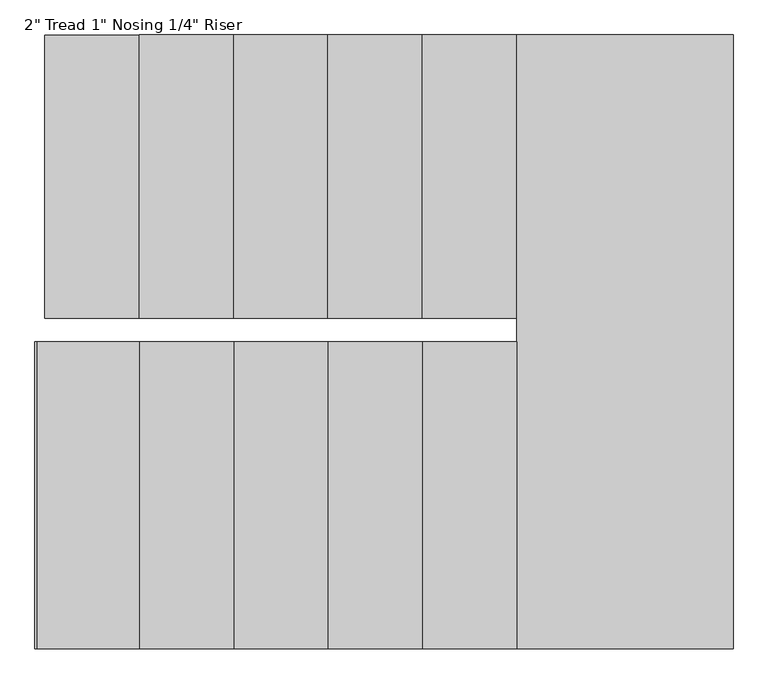
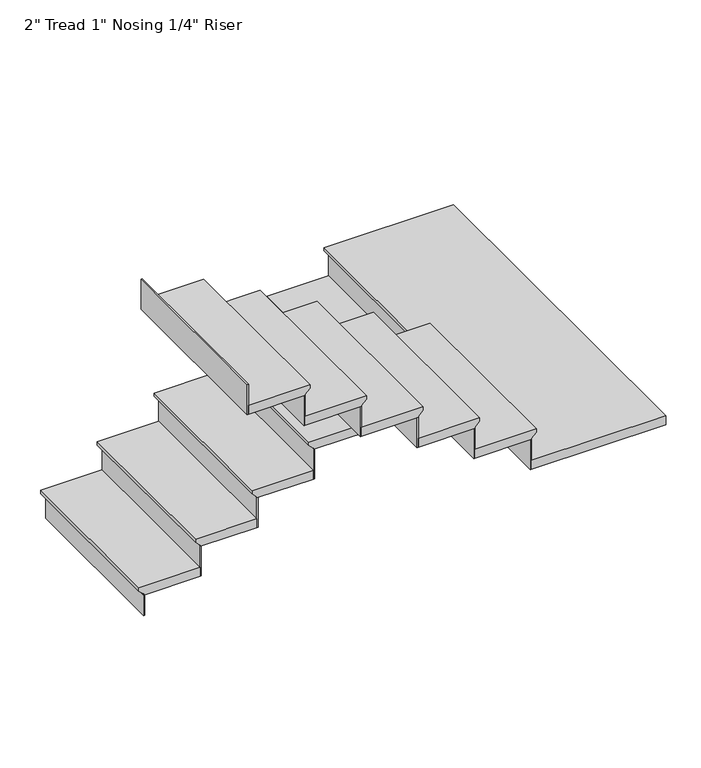
"""IFC4 building model written with IfcOpenShell, lengths in millimetres: stair flight geometry."""

from ifc_helpers import new_model, si_unit, origin, place, context, project, spatial, faceted_brep, source, transform, mapped, element, save


def stair_flight_f370bc99(model_context):
    return source(origin(), model_context, "Body", "Brep", [
        faceted_brep([(-1179.0415084, -2827.3064015, 6551.0833333), (-1179.0415084, -2827.3064015, 6570.1333333), (-1179.0415084, -1912.9064015, 6570.1333333), (-1179.0415084, -1912.9064015, 6551.0833333), (-1153.6415084, -2827.3064015, 6525.6833333), (-1153.6415084, -1912.9064015, 6525.6833333), (-848.8415084, -2827.3064015, 6570.1333333), (-848.8415084, -1912.9064015, 6570.1333333), (-1153.6415084, -1912.9064015, 6519.3333333), (-848.8415084, -1912.9064015, 6519.3333333), (-848.8415084, -2827.3064015, 6519.3333333), (-1153.6415084, -2827.3064015, 6519.3333333)], [[[0, 1, 2, 3]], [[4, 0, 3, 5]], [[2, 1, 6, 7]], [[8, 9, 10, 11]], [[2, 7, 9, 8, 5, 3]], [[8, 11, 4, 5]], [[6, 1, 0, 4, 11, 10]], [[7, 6, 10, 9]]]),
        faceted_brep([(-1153.6415084, -2827.3064015, 6519.3333333), (-1153.6415084, -2827.3064015, 6400.8), (-1147.2915084, -2827.3064015, 6400.8), (-1147.2915084, -2827.3064015, 6519.3333333), (-1153.6415084, -1912.9064015, 6519.3333333), (-1147.2915084, -1912.9064015, 6519.3333333), (-1147.2915084, -1912.9064015, 6400.8), (-1153.6415084, -1912.9064015, 6400.8)], [[[0, 1, 2, 3]], [[4, 5, 6, 7]], [[1, 0, 4, 7]], [[2, 1, 7, 6]], [[3, 2, 6, 5]], [[0, 3, 5, 4]]]),
        faceted_brep([(-848.8415084, -2827.3064015, 6688.6666667), (-848.8415084, -2827.3064015, 6519.3333333), (-842.4915084, -2827.3064015, 6519.3333333), (-842.4915084, -2827.3064015, 6688.6666667), (-848.8415084, -1912.9064015, 6688.6666667), (-842.4915084, -1912.9064015, 6688.6666667), (-842.4915084, -1912.9064015, 6519.3333333), (-848.8415084, -1912.9064015, 6519.3333333)], [[[0, 1, 2, 3]], [[4, 5, 6, 7]], [[1, 0, 4, 7]], [[2, 1, 7, 6]], [[3, 2, 6, 5]], [[0, 3, 5, 4]]]),
        faceted_brep([(-874.2415084, -1912.9064015, 6739.4666667), (-874.2415084, -2827.3064015, 6739.4666667), (-544.0415084, -2827.3064015, 6739.4666667), (-544.0415084, -1912.9064015, 6739.4666667), (-848.8415084, -1912.9064015, 6688.6666667), (-544.0415084, -1912.9064015, 6688.6666667), (-544.0415084, -2827.3064015, 6688.6666667), (-848.8415084, -2827.3064015, 6688.6666667), (-848.8415084, -1912.9064015, 6695.0166667), (-874.2415084, -1912.9064015, 6720.4166667), (-848.8415084, -2827.3064015, 6695.0166667), (-874.2415084, -2827.3064015, 6720.4166667)], [[[0, 1, 2, 3]], [[4, 5, 6, 7]], [[0, 3, 5, 4, 8, 9]], [[4, 7, 10, 8]], [[2, 1, 11, 10, 7, 6]], [[3, 2, 6, 5]], [[11, 1, 0, 9]], [[10, 11, 9, 8]]]),
        faceted_brep([(-544.0415084, -2827.3064015, 6858.0), (-544.0415084, -2827.3064015, 6688.6666667), (-537.6915084, -2827.3064015, 6688.6666667), (-537.6915084, -2827.3064015, 6858.0), (-544.0415084, -1912.9064015, 6858.0), (-537.6915084, -1912.9064015, 6858.0), (-537.6915084, -1912.9064015, 6688.6666667), (-544.0415084, -1912.9064015, 6688.6666667)], [[[0, 1, 2, 3]], [[4, 5, 6, 7]], [[1, 0, 4, 7]], [[2, 1, 7, 6]], [[3, 2, 6, 5]], [[0, 3, 5, 4]]]),
        faceted_brep([(-569.4415084, -1912.9064015, 6908.8), (-569.4415084, -2827.3064015, 6908.8), (-239.2415084, -2827.3064015, 6908.8), (-239.2415084, -1912.9064015, 6908.8), (-544.0415084, -1912.9064015, 6858.0), (-239.2415084, -1912.9064015, 6858.0), (-239.2415084, -2827.3064015, 6858.0), (-544.0415084, -2827.3064015, 6858.0), (-544.0415084, -1912.9064015, 6864.35), (-569.4415084, -1912.9064015, 6889.75), (-544.0415084, -2827.3064015, 6864.35), (-569.4415084, -2827.3064015, 6889.75)], [[[0, 1, 2, 3]], [[4, 5, 6, 7]], [[0, 3, 5, 4, 8, 9]], [[4, 7, 10, 8]], [[2, 1, 11, 10, 7, 6]], [[3, 2, 6, 5]], [[11, 1, 0, 9]], [[10, 11, 9, 8]]]),
        faceted_brep([(-239.2415084, -2827.3064015, 7027.3333333), (-239.2415084, -2827.3064015, 6858.0), (-232.8915084, -2827.3064015, 6858.0), (-232.8915084, -2827.3064015, 7027.3333333), (-239.2415084, -1912.9064015, 7027.3333333), (-232.8915084, -1912.9064015, 7027.3333333), (-232.8915084, -1912.9064015, 6858.0), (-239.2415084, -1912.9064015, 6858.0)], [[[0, 1, 2, 3]], [[4, 5, 6, 7]], [[1, 0, 4, 7]], [[2, 1, 7, 6]], [[3, 2, 6, 5]], [[0, 3, 5, 4]]]),
        faceted_brep([(-264.6415084, -1912.9064015, 7078.1333333), (-264.6415084, -2827.3064015, 7078.1333333), (65.5584916, -2827.3064015, 7078.1333333), (65.5584916, -1912.9064015, 7078.1333333), (-239.2415084, -1912.9064015, 7027.3333333), (65.5584916, -1912.9064015, 7027.3333333), (65.5584916, -2827.3064015, 7027.3333333), (-239.2415084, -2827.3064015, 7027.3333333), (-239.2415084, -1912.9064015, 7033.6833333), (-264.6415084, -1912.9064015, 7059.0833333), (-239.2415084, -2827.3064015, 7033.6833333), (-264.6415084, -2827.3064015, 7059.0833333)], [[[0, 1, 2, 3]], [[4, 5, 6, 7]], [[0, 3, 5, 4, 8, 9]], [[4, 7, 10, 8]], [[2, 1, 11, 10, 7, 6]], [[3, 2, 6, 5]], [[11, 1, 0, 9]], [[10, 11, 9, 8]]]),
        faceted_brep([(65.5584916, -2827.3064015, 7196.6666667), (65.5584916, -2827.3064015, 7027.3333333), (71.9084916, -2827.3064015, 7027.3333333), (71.9084916, -2827.3064015, 7196.6666667), (65.5584916, -1912.9064015, 7196.6666667), (71.9084916, -1912.9064015, 7196.6666667), (71.9084916, -1912.9064015, 7027.3333333), (65.5584916, -1912.9064015, 7027.3333333)], [[[0, 1, 2, 3]], [[4, 5, 6, 7]], [[1, 0, 4, 7]], [[2, 1, 7, 6]], [[3, 2, 6, 5]], [[0, 3, 5, 4]]]),
        faceted_brep([(40.1584916, -1912.9064015, 7247.4666667), (40.1584916, -2827.3064015, 7247.4666667), (370.3584916, -2827.3064015, 7247.4666667), (370.3584916, -1912.9064015, 7247.4666667), (65.5584916, -1912.9064015, 7196.6666667), (370.3584916, -1912.9064015, 7196.6666667), (370.3584916, -2827.3064015, 7196.6666667), (65.5584916, -2827.3064015, 7196.6666667), (65.5584916, -1912.9064015, 7203.0166667), (40.1584916, -1912.9064015, 7228.4166667), (65.5584916, -2827.3064015, 7203.0166667), (40.1584916, -2827.3064015, 7228.4166667)], [[[0, 1, 2, 3]], [[4, 5, 6, 7]], [[0, 3, 5, 4, 8, 9]], [[4, 7, 10, 8]], [[2, 1, 11, 10, 7, 6]], [[3, 2, 6, 5]], [[11, 1, 0, 9]], [[10, 11, 9, 8]]]),
        faceted_brep([(370.3584916, -2827.3064015, 7366.0), (370.3584916, -2827.3064015, 7196.6666667), (376.7084916, -2827.3064015, 7196.6666667), (376.7084916, -2827.3064015, 7366.0), (370.3584916, -1912.9064015, 7366.0), (376.7084916, -1912.9064015, 7366.0), (376.7084916, -1912.9064015, 7196.6666667), (370.3584916, -1912.9064015, 7196.6666667)], [[[0, 1, 2, 3]], [[4, 5, 6, 7]], [[1, 0, 4, 7]], [[2, 1, 7, 6]], [[3, 2, 6, 5]], [[0, 3, 5, 4]]]),
        faceted_brep([(319.5584916, -3894.1064015, 7416.8), (1043.4584916, -3894.1064015, 7416.8), (1043.4584916, -1912.9064015, 7416.8), (344.9584916, -1912.9064015, 7416.8), (344.9584916, -2903.5064015, 7416.8), (319.5584916, -2903.5064015, 7416.8), (1043.4584916, -3894.1064015, 7366.0), (319.5584916, -3894.1064015, 7366.0), (319.5584916, -2903.5064015, 7366.0), (344.9584916, -2903.5064015, 7366.0), (344.9584916, -2827.3064015, 7366.0), (370.3584916, -2827.3064015, 7366.0), (370.3584916, -1912.9064015, 7366.0), (1043.4584916, -1912.9064015, 7366.0), (370.3584916, -1912.9064015, 7372.35), (344.9584916, -1912.9064015, 7397.75), (370.3584916, -2827.3064015, 7372.35), (344.9584916, -2827.3064015, 7397.75)], [[[0, 1, 2, 3, 4, 5]], [[6, 7, 8, 9, 10, 11, 12, 13]], [[1, 0, 7, 6]], [[2, 1, 6, 13]], [[3, 2, 13, 12, 14, 15]], [[12, 11, 16, 14]], [[11, 10, 17, 16]], [[4, 3, 15, 17, 10, 9]], [[5, 4, 9, 8]], [[0, 5, 8, 7]], [[15, 14, 16, 17]]]),
        faceted_brep([(319.5584916, -2903.5064015, 7535.3333333), (319.5584916, -2903.5064015, 7366.0), (313.2084916, -2903.5064015, 7366.0), (313.2084916, -2903.5064015, 7535.3333333), (319.5584916, -3894.1064015, 7535.3333333), (313.2084916, -3894.1064015, 7535.3333333), (313.2084916, -3894.1064015, 7366.0), (319.5584916, -3894.1064015, 7366.0)], [[[0, 1, 2, 3]], [[4, 5, 6, 7]], [[1, 0, 4, 7]], [[2, 1, 7, 6]], [[3, 2, 6, 5]], [[0, 3, 5, 4]]]),
        faceted_brep([(344.9584916, -3894.1064015, 7586.1333333), (344.9584916, -2903.5064015, 7586.1333333), (14.7584916, -2903.5064015, 7586.1333333), (14.7584916, -3894.1064015, 7586.1333333), (319.5584916, -3894.1064015, 7535.3333333), (14.7584916, -3894.1064015, 7535.3333333), (14.7584916, -2903.5064015, 7535.3333333), (319.5584916, -2903.5064015, 7535.3333333), (319.5584916, -3894.1064015, 7541.6833333), (344.9584916, -3894.1064015, 7567.0833333), (319.5584916, -2903.5064015, 7541.6833333), (344.9584916, -2903.5064015, 7567.0833333)], [[[0, 1, 2, 3]], [[4, 5, 6, 7]], [[0, 3, 5, 4, 8, 9]], [[4, 7, 10, 8]], [[2, 1, 11, 10, 7, 6]], [[3, 2, 6, 5]], [[11, 1, 0, 9]], [[10, 11, 9, 8]]]),
        faceted_brep([(14.7584916, -2903.5064015, 7704.6666667), (14.7584916, -2903.5064015, 7535.3333333), (8.4084916, -2903.5064015, 7535.3333333), (8.4084916, -2903.5064015, 7704.6666667), (14.7584916, -3894.1064015, 7704.6666667), (8.4084916, -3894.1064015, 7704.6666667), (8.4084916, -3894.1064015, 7535.3333333), (14.7584916, -3894.1064015, 7535.3333333)], [[[0, 1, 2, 3]], [[4, 5, 6, 7]], [[1, 0, 4, 7]], [[2, 1, 7, 6]], [[3, 2, 6, 5]], [[0, 3, 5, 4]]]),
        faceted_brep([(40.1584916, -3894.1064015, 7755.4666667), (40.1584916, -2903.5064015, 7755.4666667), (-290.0415084, -2903.5064015, 7755.4666667), (-290.0415084, -3894.1064015, 7755.4666667), (14.7584916, -3894.1064015, 7704.6666667), (-290.0415084, -3894.1064015, 7704.6666667), (-290.0415084, -2903.5064015, 7704.6666667), (14.7584916, -2903.5064015, 7704.6666667), (14.7584916, -3894.1064015, 7711.0166667), (40.1584916, -3894.1064015, 7736.4166667), (14.7584916, -2903.5064015, 7711.0166667), (40.1584916, -2903.5064015, 7736.4166667)], [[[0, 1, 2, 3]], [[4, 5, 6, 7]], [[0, 3, 5, 4, 8, 9]], [[4, 7, 10, 8]], [[2, 1, 11, 10, 7, 6]], [[3, 2, 6, 5]], [[11, 1, 0, 9]], [[10, 11, 9, 8]]]),
        faceted_brep([(-290.0415084, -2903.5064015, 7874.0), (-290.0415084, -2903.5064015, 7704.6666667), (-296.3915084, -2903.5064015, 7704.6666667), (-296.3915084, -2903.5064015, 7874.0), (-290.0415084, -3894.1064015, 7874.0), (-296.3915084, -3894.1064015, 7874.0), (-296.3915084, -3894.1064015, 7704.6666667), (-290.0415084, -3894.1064015, 7704.6666667)], [[[0, 1, 2, 3]], [[4, 5, 6, 7]], [[1, 0, 4, 7]], [[2, 1, 7, 6]], [[3, 2, 6, 5]], [[0, 3, 5, 4]]]),
        faceted_brep([(-264.6415084, -3894.1064015, 7924.8), (-264.6415084, -2903.5064015, 7924.8), (-594.8415084, -2903.5064015, 7924.8), (-594.8415084, -3894.1064015, 7924.8), (-290.0415084, -3894.1064015, 7874.0), (-594.8415084, -3894.1064015, 7874.0), (-594.8415084, -2903.5064015, 7874.0), (-290.0415084, -2903.5064015, 7874.0), (-290.0415084, -3894.1064015, 7880.35), (-264.6415084, -3894.1064015, 7905.75), (-290.0415084, -2903.5064015, 7880.35), (-264.6415084, -2903.5064015, 7905.75)], [[[0, 1, 2, 3]], [[4, 5, 6, 7]], [[0, 3, 5, 4, 8, 9]], [[4, 7, 10, 8]], [[2, 1, 11, 10, 7, 6]], [[3, 2, 6, 5]], [[11, 1, 0, 9]], [[10, 11, 9, 8]]]),
        faceted_brep([(-594.8415084, -2903.5064015, 8043.3333333), (-594.8415084, -2903.5064015, 7874.0), (-601.1915084, -2903.5064015, 7874.0), (-601.1915084, -2903.5064015, 8043.3333333), (-594.8415084, -3894.1064015, 8043.3333333), (-601.1915084, -3894.1064015, 8043.3333333), (-601.1915084, -3894.1064015, 7874.0), (-594.8415084, -3894.1064015, 7874.0)], [[[0, 1, 2, 3]], [[4, 5, 6, 7]], [[1, 0, 4, 7]], [[2, 1, 7, 6]], [[3, 2, 6, 5]], [[0, 3, 5, 4]]]),
        faceted_brep([(-569.4415084, -3894.1064015, 8094.1333333), (-569.4415084, -2903.5064015, 8094.1333333), (-899.6415084, -2903.5064015, 8094.1333333), (-899.6415084, -3894.1064015, 8094.1333333), (-594.8415084, -3894.1064015, 8043.3333333), (-899.6415084, -3894.1064015, 8043.3333333), (-899.6415084, -2903.5064015, 8043.3333333), (-594.8415084, -2903.5064015, 8043.3333333), (-594.8415084, -3894.1064015, 8049.6833333), (-569.4415084, -3894.1064015, 8075.0833333), (-594.8415084, -2903.5064015, 8049.6833333), (-569.4415084, -2903.5064015, 8075.0833333)], [[[0, 1, 2, 3]], [[4, 5, 6, 7]], [[0, 3, 5, 4, 8, 9]], [[4, 7, 10, 8]], [[2, 1, 11, 10, 7, 6]], [[3, 2, 6, 5]], [[11, 1, 0, 9]], [[10, 11, 9, 8]]]),
        faceted_brep([(-899.6415084, -2903.5064015, 8212.6666667), (-899.6415084, -2903.5064015, 8043.3333333), (-905.9915084, -2903.5064015, 8043.3333333), (-905.9915084, -2903.5064015, 8212.6666667), (-899.6415084, -3894.1064015, 8212.6666667), (-905.9915084, -3894.1064015, 8212.6666667), (-905.9915084, -3894.1064015, 8043.3333333), (-899.6415084, -3894.1064015, 8043.3333333)], [[[0, 1, 2, 3]], [[4, 5, 6, 7]], [[1, 0, 4, 7]], [[2, 1, 7, 6]], [[3, 2, 6, 5]], [[0, 3, 5, 4]]]),
        faceted_brep([(-1204.4415084, -2903.5064015, 8382.0), (-1204.4415084, -2903.5064015, 8212.6666667), (-1210.7915084, -2903.5064015, 8212.6666667), (-1210.7915084, -2903.5064015, 8382.0), (-1204.4415084, -3894.1064015, 8382.0), (-1210.7915084, -3894.1064015, 8382.0), (-1210.7915084, -3894.1064015, 8212.6666667), (-1204.4415084, -3894.1064015, 8212.6666667)], [[[0, 1, 2, 3]], [[4, 5, 6, 7]], [[1, 0, 4, 7]], [[2, 1, 7, 6]], [[3, 2, 6, 5]], [[0, 3, 5, 4]]]),
        faceted_brep([(-874.2415084, -3894.1064015, 8263.4666667), (-874.2415084, -2903.5064015, 8263.4666667), (-1204.4415084, -2903.5064015, 8263.4666667), (-1204.4415084, -3894.1064015, 8263.4666667), (-899.6415084, -3894.1064015, 8212.6666667), (-1204.4415084, -3894.1064015, 8212.6666667), (-1204.4415084, -2903.5064015, 8212.6666667), (-899.6415084, -2903.5064015, 8212.6666667), (-899.6415084, -3894.1064015, 8219.0166667), (-874.2415084, -3894.1064015, 8244.4166667), (-899.6415084, -2903.5064015, 8219.0166667), (-874.2415084, -2903.5064015, 8244.4166667)], [[[0, 1, 2, 3]], [[4, 5, 6, 7]], [[0, 3, 5, 4, 8, 9]], [[4, 7, 10, 8]], [[2, 1, 11, 10, 7, 6]], [[3, 2, 6, 5]], [[11, 1, 0, 9]], [[10, 11, 9, 8]]]),
    ])


if __name__ == "__main__":
    model = new_model("IFC4")
    model_context = context("Model", 3, world=origin())
    ifc_project = project(units=[si_unit("LENGTHUNIT", "METRE", prefix="MILLI")], contexts=[model_context])
    site = spatial("IfcSite", under=ifc_project)
    building = spatial("IfcBuilding", under=site)
    placement = place(None, origin())
    stair_flight_shape = stair_flight_f370bc99(model_context)
    element("IfcStairFlight", 1, ObjectType="2\" Tread 1\" Nosing 1/4\" Riser", at=placement, inside=building, context=model_context, shape_type="MappedRepresentation", body=[
        mapped(stair_flight_shape, transform((0.0, 0.0, 0.0), x_axis=(1.0, 0.0, 0.0), y_axis=(0.0, 1.0, 0.0), z_axis=(0.0, 0.0, 1.0))),
    ])
    save(model, "model.ifc")
